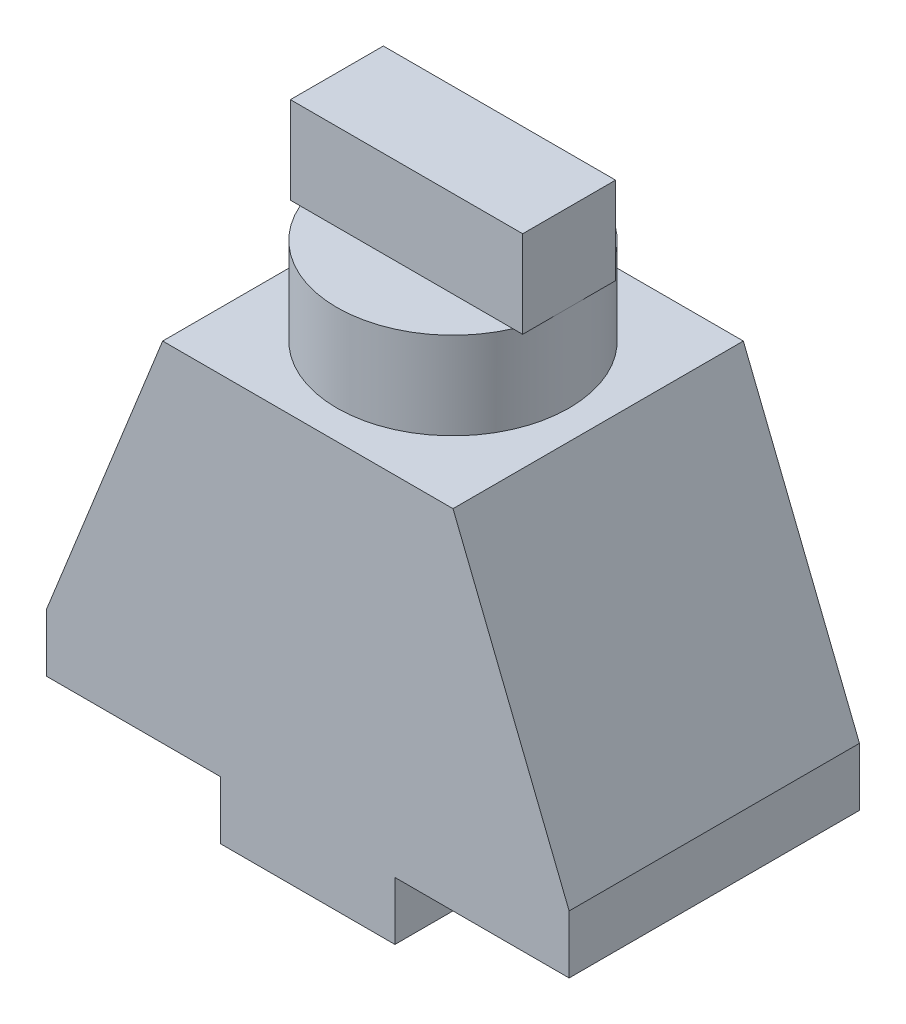
ISO-10303-21;
HEADER;
FILE_DESCRIPTION(('STEP AP214'),'2;1');
FILE_NAME('part.step','',(''),(''),'','','');
FILE_SCHEMA(('AUTOMOTIVE_DESIGN { 1 0 10303 214 1 1 1 1 }'));
ENDSEC;
DATA;
#1=APPLICATION_CONTEXT('core data for automotive mechanical design processes');
#2=APPLICATION_PROTOCOL_DEFINITION('international standard','automotive_design',2000,#1);
#3=PRODUCT_CONTEXT('',#1,'mechanical');
#4=PRODUCT('Part','Part','',(#3));
#5=PRODUCT_RELATED_PRODUCT_CATEGORY('part','',(#4));
#6=PRODUCT_DEFINITION_FORMATION('','',#4);
#7=PRODUCT_DEFINITION_CONTEXT('part definition',#1,'design');
#8=PRODUCT_DEFINITION('design','',#6,#7);
#9=PRODUCT_DEFINITION_SHAPE('','',#8);
#10=(LENGTH_UNIT() NAMED_UNIT(*) SI_UNIT(.MILLI.,.METRE.));
#11=(NAMED_UNIT(*) PLANE_ANGLE_UNIT() SI_UNIT($,.RADIAN.));
#12=(NAMED_UNIT(*) SI_UNIT($,.STERADIAN.) SOLID_ANGLE_UNIT());
#13=UNCERTAINTY_MEASURE_WITH_UNIT(LENGTH_MEASURE(1.E-05),#10,'distance_accuracy_value','');
#14=(GEOMETRIC_REPRESENTATION_CONTEXT(3) GLOBAL_UNCERTAINTY_ASSIGNED_CONTEXT((#13)) GLOBAL_UNIT_ASSIGNED_CONTEXT((#10,
#11,#12)) REPRESENTATION_CONTEXT('',''));
#15=CARTESIAN_POINT('',(0.,0.,0.));
#16=DIRECTION('',(0.,0.,1.));
#17=DIRECTION('',(1.,0.,0.));
#18=AXIS2_PLACEMENT_3D('',#15,#16,#17);
#19=CARTESIAN_POINT('',(0.,70.,25.));
#20=DIRECTION('',(0.,1.,0.));
#21=DIRECTION('',(0.,0.,1.));
#22=AXIS2_PLACEMENT_3D('',#19,#20,#21);
#23=PLANE('',#22);
#24=DIRECTION('',(1.,0.,0.));
#25=VECTOR('',#24,1.);
#26=CARTESIAN_POINT('',(-20.,70.,33.));
#27=LINE('',#26,#25);
#28=CARTESIAN_POINT('',(-18.3303027798234,70.,33.));
#29=VERTEX_POINT('',#28);
#30=CARTESIAN_POINT('',(18.3303027798234,70.,33.));
#31=VERTEX_POINT('',#30);
#32=EDGE_CURVE('E12',#29,#31,#27,.T.);
#33=ORIENTED_EDGE('',*,*,#32,.F.);
#34=CARTESIAN_POINT('',(0.,70.,25.));
#35=DIRECTION('',(0.,1.,0.));
#36=DIRECTION('',(0.,0.,1.));
#37=AXIS2_PLACEMENT_3D('',#34,#35,#36);
#38=CIRCLE('',#37,20.);
#39=EDGE_CURVE('E267',#29,#31,#38,.T.);
#40=ORIENTED_EDGE('',*,*,#39,.T.);
#41=EDGE_LOOP('',(#33,#40));
#42=FACE_BOUND('',#41,.T.);
#43=ADVANCED_FACE('F47',(#42),#23,.T.);
#44=CARTESIAN_POINT('',(45.,5.,50.));
#45=DIRECTION('',(-1.,0.,0.));
#46=DIRECTION('',(0.,0.,1.));
#47=AXIS2_PLACEMENT_3D('',#44,#45,#46);
#48=PLANE('',#47);
#49=DIRECTION('',(0.,1.,0.));
#50=VECTOR('',#49,1.);
#51=CARTESIAN_POINT('',(45.,5.,0.));
#52=LINE('',#51,#50);
#53=CARTESIAN_POINT('',(45.,-5.,0.));
#54=VERTEX_POINT('',#53);
#55=CARTESIAN_POINT('',(45.,5.00000000000001,0.));
#56=VERTEX_POINT('',#55);
#57=EDGE_CURVE('E355',#54,#56,#52,.T.);
#58=ORIENTED_EDGE('',*,*,#57,.T.);
#59=DIRECTION('',(0.,0.,1.));
#60=VECTOR('',#59,1.);
#61=CARTESIAN_POINT('',(45.,5.00000000000001,0.));
#62=LINE('',#61,#60);
#63=CARTESIAN_POINT('',(45.,5.00000000000001,50.));
#64=VERTEX_POINT('',#63);
#65=EDGE_CURVE('E273',#64,#56,#62,.F.);
#66=ORIENTED_EDGE('',*,*,#65,.F.);
#67=DIRECTION('',(0.,1.,0.));
#68=VECTOR('',#67,1.);
#69=CARTESIAN_POINT('',(45.,5.,50.));
#70=LINE('',#69,#68);
#71=CARTESIAN_POINT('',(45.,-5.,50.));
#72=VERTEX_POINT('',#71);
#73=EDGE_CURVE('E358',#72,#64,#70,.T.);
#74=ORIENTED_EDGE('',*,*,#73,.F.);
#75=DIRECTION('',(0.,0.,-1.));
#76=VECTOR('',#75,1.);
#77=CARTESIAN_POINT('',(45.,-5.,50.));
#78=LINE('',#77,#76);
#79=EDGE_CURVE('E446',#72,#54,#78,.T.);
#80=ORIENTED_EDGE('',*,*,#79,.T.);
#81=EDGE_LOOP('',(#58,#66,#74,#80));
#82=FACE_BOUND('',#81,.T.);
#83=ADVANCED_FACE('F51',(#82),#48,.F.);
#84=CARTESIAN_POINT('',(-45.,5.,50.));
#85=DIRECTION('',(1.,0.,0.));
#86=DIRECTION('',(0.,0.,-1.));
#87=AXIS2_PLACEMENT_3D('',#84,#85,#86);
#88=PLANE('',#87);
#89=DIRECTION('',(0.,-1.,0.));
#90=VECTOR('',#89,1.);
#91=CARTESIAN_POINT('',(-45.,5.,0.));
#92=LINE('',#91,#90);
#93=CARTESIAN_POINT('',(-45.,5.,0.));
#94=VERTEX_POINT('',#93);
#95=CARTESIAN_POINT('',(-45.,-5.,0.));
#96=VERTEX_POINT('',#95);
#97=EDGE_CURVE('E347',#94,#96,#92,.T.);
#98=ORIENTED_EDGE('',*,*,#97,.T.);
#99=DIRECTION('',(0.,0.,-1.));
#100=VECTOR('',#99,1.);
#101=CARTESIAN_POINT('',(-45.,-5.,50.));
#102=LINE('',#101,#100);
#103=CARTESIAN_POINT('',(-45.,-5.,50.));
#104=VERTEX_POINT('',#103);
#105=EDGE_CURVE('E333',#104,#96,#102,.T.);
#106=ORIENTED_EDGE('',*,*,#105,.F.);
#107=DIRECTION('',(0.,-1.,0.));
#108=VECTOR('',#107,1.);
#109=CARTESIAN_POINT('',(-45.,5.,50.));
#110=LINE('',#109,#108);
#111=CARTESIAN_POINT('',(-45.,4.99999999999999,50.));
#112=VERTEX_POINT('',#111);
#113=EDGE_CURVE('E353',#112,#104,#110,.T.);
#114=ORIENTED_EDGE('',*,*,#113,.F.);
#115=DIRECTION('',(0.,0.,-1.));
#116=VECTOR('',#115,1.);
#117=CARTESIAN_POINT('',(-45.,5.,50.));
#118=LINE('',#117,#116);
#119=EDGE_CURVE('E52',#112,#94,#118,.T.);
#120=ORIENTED_EDGE('',*,*,#119,.T.);
#121=EDGE_LOOP('',(#98,#106,#114,#120));
#122=FACE_BOUND('',#121,.T.);
#123=ADVANCED_FACE('F492',(#122),#88,.F.);
#124=CARTESIAN_POINT('',(-45.,-5.,50.));
#125=DIRECTION('',(0.,1.,0.));
#126=DIRECTION('',(0.,0.,1.));
#127=AXIS2_PLACEMENT_3D('',#124,#125,#126);
#128=PLANE('',#127);
#129=DIRECTION('',(1.,0.,0.));
#130=VECTOR('',#129,1.);
#131=CARTESIAN_POINT('',(-45.,-5.,0.));
#132=LINE('',#131,#130);
#133=CARTESIAN_POINT('',(-15.,-5.,0.));
#134=VERTEX_POINT('',#133);
#135=EDGE_CURVE('E352',#96,#134,#132,.T.);
#136=ORIENTED_EDGE('',*,*,#135,.T.);
#137=DIRECTION('',(0.,0.,-1.));
#138=VECTOR('',#137,1.);
#139=CARTESIAN_POINT('',(-15.,-5.,50.));
#140=LINE('',#139,#138);
#141=CARTESIAN_POINT('',(-15.,-5.,50.));
#142=VERTEX_POINT('',#141);
#143=EDGE_CURVE('E336',#142,#134,#140,.T.);
#144=ORIENTED_EDGE('',*,*,#143,.F.);
#145=DIRECTION('',(1.,0.,0.));
#146=VECTOR('',#145,1.);
#147=CARTESIAN_POINT('',(-45.,-5.,50.));
#148=LINE('',#147,#146);
#149=EDGE_CURVE('E351',#104,#142,#148,.T.);
#150=ORIENTED_EDGE('',*,*,#149,.F.);
#151=ORIENTED_EDGE('',*,*,#105,.T.);
#152=EDGE_LOOP('',(#136,#144,#150,#151));
#153=FACE_BOUND('',#152,.T.);
#154=ADVANCED_FACE('F481',(#153),#128,.F.);
#155=CARTESIAN_POINT('',(-15.,-5.,50.));
#156=DIRECTION('',(1.,0.,0.));
#157=DIRECTION('',(0.,0.,-1.));
#158=AXIS2_PLACEMENT_3D('',#155,#156,#157);
#159=PLANE('',#158);
#160=DIRECTION('',(0.,-1.,0.));
#161=VECTOR('',#160,1.);
#162=CARTESIAN_POINT('',(-15.,-5.,0.));
#163=LINE('',#162,#161);
#164=CARTESIAN_POINT('',(-15.,-15.,0.));
#165=VERTEX_POINT('',#164);
#166=EDGE_CURVE('E476',#134,#165,#163,.T.);
#167=ORIENTED_EDGE('',*,*,#166,.T.);
#168=DIRECTION('',(0.,0.,-1.));
#169=VECTOR('',#168,1.);
#170=CARTESIAN_POINT('',(-15.,-15.,50.));
#171=LINE('',#170,#169);
#172=CARTESIAN_POINT('',(-15.,-15.,50.));
#173=VERTEX_POINT('',#172);
#174=EDGE_CURVE('E343',#173,#165,#171,.T.);
#175=ORIENTED_EDGE('',*,*,#174,.F.);
#176=DIRECTION('',(0.,-1.,0.));
#177=VECTOR('',#176,1.);
#178=CARTESIAN_POINT('',(-15.,-5.,50.));
#179=LINE('',#178,#177);
#180=EDGE_CURVE('E483',#142,#173,#179,.T.);
#181=ORIENTED_EDGE('',*,*,#180,.F.);
#182=ORIENTED_EDGE('',*,*,#143,.T.);
#183=EDGE_LOOP('',(#167,#175,#181,#182));
#184=FACE_BOUND('',#183,.T.);
#185=ADVANCED_FACE('F488',(#184),#159,.F.);
#186=CARTESIAN_POINT('',(-15.,-15.,50.));
#187=DIRECTION('',(0.,1.,0.));
#188=DIRECTION('',(0.,0.,1.));
#189=AXIS2_PLACEMENT_3D('',#186,#187,#188);
#190=PLANE('',#189);
#191=DIRECTION('',(1.,0.,0.));
#192=VECTOR('',#191,1.);
#193=CARTESIAN_POINT('',(-15.,-15.,0.));
#194=LINE('',#193,#192);
#195=CARTESIAN_POINT('',(15.,-15.,0.));
#196=VERTEX_POINT('',#195);
#197=EDGE_CURVE('E460',#165,#196,#194,.T.);
#198=ORIENTED_EDGE('',*,*,#197,.T.);
#199=DIRECTION('',(0.,0.,-1.));
#200=VECTOR('',#199,1.);
#201=CARTESIAN_POINT('',(15.,-15.,50.));
#202=LINE('',#201,#200);
#203=CARTESIAN_POINT('',(15.,-15.,50.));
#204=VERTEX_POINT('',#203);
#205=EDGE_CURVE('E464',#204,#196,#202,.T.);
#206=ORIENTED_EDGE('',*,*,#205,.F.);
#207=DIRECTION('',(1.,0.,0.));
#208=VECTOR('',#207,1.);
#209=CARTESIAN_POINT('',(-15.,-15.,50.));
#210=LINE('',#209,#208);
#211=EDGE_CURVE('E475',#173,#204,#210,.T.);
#212=ORIENTED_EDGE('',*,*,#211,.F.);
#213=ORIENTED_EDGE('',*,*,#174,.T.);
#214=EDGE_LOOP('',(#198,#206,#212,#213));
#215=FACE_BOUND('',#214,.T.);
#216=ADVANCED_FACE('F468',(#215),#190,.F.);
#217=CARTESIAN_POINT('',(15.,-5.,50.));
#218=DIRECTION('',(-1.,0.,0.));
#219=DIRECTION('',(0.,0.,1.));
#220=AXIS2_PLACEMENT_3D('',#217,#218,#219);
#221=PLANE('',#220);
#222=DIRECTION('',(0.,1.,0.));
#223=VECTOR('',#222,1.);
#224=CARTESIAN_POINT('',(15.,-5.,0.));
#225=LINE('',#224,#223);
#226=CARTESIAN_POINT('',(15.,-5.,0.));
#227=VERTEX_POINT('',#226);
#228=EDGE_CURVE('E454',#196,#227,#225,.T.);
#229=ORIENTED_EDGE('',*,*,#228,.T.);
#230=DIRECTION('',(0.,0.,-1.));
#231=VECTOR('',#230,1.);
#232=CARTESIAN_POINT('',(15.,-5.,50.));
#233=LINE('',#232,#231);
#234=CARTESIAN_POINT('',(15.,-5.,50.));
#235=VERTEX_POINT('',#234);
#236=EDGE_CURVE('E465',#235,#227,#233,.T.);
#237=ORIENTED_EDGE('',*,*,#236,.F.);
#238=DIRECTION('',(0.,1.,0.));
#239=VECTOR('',#238,1.);
#240=CARTESIAN_POINT('',(15.,-5.,50.));
#241=LINE('',#240,#239);
#242=EDGE_CURVE('E482',#204,#235,#241,.T.);
#243=ORIENTED_EDGE('',*,*,#242,.F.);
#244=ORIENTED_EDGE('',*,*,#205,.T.);
#245=EDGE_LOOP('',(#229,#237,#243,#244));
#246=FACE_BOUND('',#245,.T.);
#247=ADVANCED_FACE('F491',(#246),#221,.F.);
#248=CARTESIAN_POINT('',(15.,-5.,50.));
#249=DIRECTION('',(0.,1.,0.));
#250=DIRECTION('',(0.,0.,1.));
#251=AXIS2_PLACEMENT_3D('',#248,#249,#250);
#252=PLANE('',#251);
#253=DIRECTION('',(1.,0.,0.));
#254=VECTOR('',#253,1.);
#255=CARTESIAN_POINT('',(15.,-5.,0.));
#256=LINE('',#255,#254);
#257=EDGE_CURVE('E360',#227,#54,#256,.T.);
#258=ORIENTED_EDGE('',*,*,#257,.T.);
#259=ORIENTED_EDGE('',*,*,#79,.F.);
#260=DIRECTION('',(1.,0.,0.));
#261=VECTOR('',#260,1.);
#262=CARTESIAN_POINT('',(15.,-5.,50.));
#263=LINE('',#262,#261);
#264=EDGE_CURVE('E444',#235,#72,#263,.T.);
#265=ORIENTED_EDGE('',*,*,#264,.F.);
#266=ORIENTED_EDGE('',*,*,#236,.T.);
#267=EDGE_LOOP('',(#258,#259,#265,#266));
#268=FACE_BOUND('',#267,.T.);
#269=ADVANCED_FACE('F317',(#268),#252,.F.);
#270=CARTESIAN_POINT('',(0.,0.,50.));
#271=DIRECTION('',(0.,0.,1.));
#272=DIRECTION('',(1.,0.,0.));
#273=AXIS2_PLACEMENT_3D('',#270,#271,#272);
#274=PLANE('',#273);
#275=ORIENTED_EDGE('',*,*,#73,.T.);
#276=DIRECTION('',(0.371390676354104,-0.928476690885259,0.));
#277=VECTOR('',#276,1.);
#278=CARTESIAN_POINT('',(25.,55.,50.));
#279=LINE('',#278,#277);
#280=CARTESIAN_POINT('',(25.,55.,50.));
#281=VERTEX_POINT('',#280);
#282=EDGE_CURVE('E282',#281,#64,#279,.T.);
#283=ORIENTED_EDGE('',*,*,#282,.F.);
#284=DIRECTION('',(1.,0.,0.));
#285=VECTOR('',#284,1.);
#286=CARTESIAN_POINT('',(-25.,55.,50.));
#287=LINE('',#286,#285);
#288=CARTESIAN_POINT('',(-25.,55.,50.));
#289=VERTEX_POINT('',#288);
#290=EDGE_CURVE('E382',#289,#281,#287,.T.);
#291=ORIENTED_EDGE('',*,*,#290,.F.);
#292=DIRECTION('',(-0.371390676354104,-0.928476690885259,0.));
#293=VECTOR('',#292,1.);
#294=CARTESIAN_POINT('',(-25.,55.,50.));
#295=LINE('',#294,#293);
#296=EDGE_CURVE('E365',#289,#112,#295,.T.);
#297=ORIENTED_EDGE('',*,*,#296,.T.);
#298=ORIENTED_EDGE('',*,*,#113,.T.);
#299=ORIENTED_EDGE('',*,*,#149,.T.);
#300=ORIENTED_EDGE('',*,*,#180,.T.);
#301=ORIENTED_EDGE('',*,*,#211,.T.);
#302=ORIENTED_EDGE('',*,*,#242,.T.);
#303=ORIENTED_EDGE('',*,*,#264,.T.);
#304=EDGE_LOOP('',(#275,#283,#291,#297,#298,#299,#300,#301,#302,#303));
#305=FACE_BOUND('',#304,.T.);
#306=ADVANCED_FACE('F311',(#305),#274,.T.);
#307=CARTESIAN_POINT('',(0.,0.,0.));
#308=DIRECTION('',(0.,0.,1.));
#309=DIRECTION('',(1.,0.,0.));
#310=AXIS2_PLACEMENT_3D('',#307,#308,#309);
#311=PLANE('',#310);
#312=ORIENTED_EDGE('',*,*,#57,.F.);
#313=ORIENTED_EDGE('',*,*,#257,.F.);
#314=ORIENTED_EDGE('',*,*,#228,.F.);
#315=ORIENTED_EDGE('',*,*,#197,.F.);
#316=ORIENTED_EDGE('',*,*,#166,.F.);
#317=ORIENTED_EDGE('',*,*,#135,.F.);
#318=ORIENTED_EDGE('',*,*,#97,.F.);
#319=DIRECTION('',(-0.371390676354103,-0.92847669088526,0.));
#320=VECTOR('',#319,1.);
#321=CARTESIAN_POINT('',(-25.,55.,0.));
#322=LINE('',#321,#320);
#323=CARTESIAN_POINT('',(-25.,55.,0.));
#324=VERTEX_POINT('',#323);
#325=EDGE_CURVE('E276',#324,#94,#322,.T.);
#326=ORIENTED_EDGE('',*,*,#325,.F.);
#327=DIRECTION('',(-1.,0.,0.));
#328=VECTOR('',#327,1.);
#329=CARTESIAN_POINT('',(-25.,55.,0.));
#330=LINE('',#329,#328);
#331=CARTESIAN_POINT('',(25.,55.,0.));
#332=VERTEX_POINT('',#331);
#333=EDGE_CURVE('E278',#332,#324,#330,.T.);
#334=ORIENTED_EDGE('',*,*,#333,.F.);
#335=DIRECTION('',(0.371390676354104,-0.928476690885259,0.));
#336=VECTOR('',#335,1.);
#337=CARTESIAN_POINT('',(25.,55.,0.));
#338=LINE('',#337,#336);
#339=EDGE_CURVE('E277',#332,#56,#338,.T.);
#340=ORIENTED_EDGE('',*,*,#339,.T.);
#341=EDGE_LOOP('',(#312,#313,#314,#315,#316,#317,#318,#326,#334,#340));
#342=FACE_BOUND('',#341,.T.);
#343=ADVANCED_FACE('F314',(#342),#311,.F.);
#344=CARTESIAN_POINT('',(0.,55.,0.));
#345=DIRECTION('',(0.,1.,0.));
#346=DIRECTION('',(0.,0.,1.));
#347=AXIS2_PLACEMENT_3D('',#344,#345,#346);
#348=PLANE('',#347);
#349=CARTESIAN_POINT('',(0.,55.,25.));
#350=DIRECTION('',(0.,1.,0.));
#351=DIRECTION('',(0.,0.,1.));
#352=AXIS2_PLACEMENT_3D('',#349,#350,#351);
#353=CIRCLE('',#352,20.);
#354=CARTESIAN_POINT('',(0.,55.,45.));
#355=VERTEX_POINT('',#354);
#356=EDGE_CURVE('E275',#355,#355,#353,.T.);
#357=ORIENTED_EDGE('',*,*,#356,.F.);
#358=EDGE_LOOP('',(#357));
#359=FACE_BOUND('',#358,.T.);
#360=DIRECTION('',(0.,0.,-1.));
#361=VECTOR('',#360,1.);
#362=CARTESIAN_POINT('',(25.,55.,0.));
#363=LINE('',#362,#361);
#364=EDGE_CURVE('E266',#281,#332,#363,.T.);
#365=ORIENTED_EDGE('',*,*,#364,.T.);
#366=ORIENTED_EDGE('',*,*,#333,.T.);
#367=DIRECTION('',(0.,0.,1.));
#368=VECTOR('',#367,1.);
#369=CARTESIAN_POINT('',(-25.,55.,0.));
#370=LINE('',#369,#368);
#371=EDGE_CURVE('E380',#324,#289,#370,.T.);
#372=ORIENTED_EDGE('',*,*,#371,.T.);
#373=ORIENTED_EDGE('',*,*,#290,.T.);
#374=EDGE_LOOP('',(#365,#366,#372,#373));
#375=FACE_BOUND('',#374,.T.);
#376=ADVANCED_FACE('F379',(#359,#375),#348,.T.);
#377=CARTESIAN_POINT('',(-40.5172413793104,16.2068965517241,0.));
#378=DIRECTION('',(0.92847669088526,-0.371390676354103,0.));
#379=DIRECTION('',(0.371390676354103,0.92847669088526,0.));
#380=AXIS2_PLACEMENT_3D('',#377,#378,#379);
#381=PLANE('',#380);
#382=DIRECTION('',(0.,0.,-1.));
#383=VECTOR('',#382,1.);
#384=CARTESIAN_POINT('',(-29.0852974398952,44.7867564002622,10.));
#385=LINE('',#384,#383);
#386=CARTESIAN_POINT('',(-29.0852974398952,44.7867564002622,40.));
#387=VERTEX_POINT('',#386);
#388=CARTESIAN_POINT('',(-29.0852974398952,44.7867564002622,10.));
#389=VERTEX_POINT('',#388);
#390=EDGE_CURVE('E223',#387,#389,#385,.T.);
#391=ORIENTED_EDGE('',*,*,#390,.F.);
#392=DIRECTION('',(0.371390676354104,0.92847669088526,0.));
#393=VECTOR('',#392,1.);
#394=CARTESIAN_POINT('',(-29.0852974398952,44.7867564002622,40.));
#395=LINE('',#394,#393);
#396=CARTESIAN_POINT('',(-39.8556270541642,17.8609323645896,40.));
#397=VERTEX_POINT('',#396);
#398=EDGE_CURVE('E68',#397,#387,#395,.T.);
#399=ORIENTED_EDGE('',*,*,#398,.F.);
#400=DIRECTION('',(0.,0.,1.));
#401=VECTOR('',#400,1.);
#402=CARTESIAN_POINT('',(-39.8556270541642,17.8609323645896,10.));
#403=LINE('',#402,#401);
#404=CARTESIAN_POINT('',(-39.8556270541642,17.8609323645896,10.));
#405=VERTEX_POINT('',#404);
#406=EDGE_CURVE('E211',#405,#397,#403,.T.);
#407=ORIENTED_EDGE('',*,*,#406,.F.);
#408=DIRECTION('',(-0.371390676354104,-0.92847669088526,0.));
#409=VECTOR('',#408,1.);
#410=CARTESIAN_POINT('',(-29.0852974398952,44.7867564002622,10.));
#411=LINE('',#410,#409);
#412=EDGE_CURVE('E220',#389,#405,#411,.T.);
#413=ORIENTED_EDGE('',*,*,#412,.F.);
#414=EDGE_LOOP('',(#391,#399,#407,#413));
#415=FACE_BOUND('',#414,.T.);
#416=ORIENTED_EDGE('',*,*,#325,.T.);
#417=ORIENTED_EDGE('',*,*,#119,.F.);
#418=ORIENTED_EDGE('',*,*,#296,.F.);
#419=ORIENTED_EDGE('',*,*,#371,.F.);
#420=EDGE_LOOP('',(#416,#417,#418,#419));
#421=FACE_BOUND('',#420,.T.);
#422=ADVANCED_FACE('F308',(#415,#421),#381,.F.);
#423=CARTESIAN_POINT('',(40.5172413793104,16.2068965517241,0.));
#424=DIRECTION('',(0.92847669088526,0.371390676354104,0.));
#425=DIRECTION('',(-0.371390676354104,0.928476690885259,0.));
#426=AXIS2_PLACEMENT_3D('',#423,#424,#425);
#427=PLANE('',#426);
#428=ORIENTED_EDGE('',*,*,#282,.T.);
#429=ORIENTED_EDGE('',*,*,#65,.T.);
#430=ORIENTED_EDGE('',*,*,#339,.F.);
#431=ORIENTED_EDGE('',*,*,#364,.F.);
#432=EDGE_LOOP('',(#428,#429,#430,#431));
#433=FACE_BOUND('',#432,.T.);
#434=ADVANCED_FACE('F300',(#433),#427,.T.);
#435=CARTESIAN_POINT('',(0.,70.,25.));
#436=DIRECTION('',(0.,-1.,0.));
#437=DIRECTION('',(0.,0.,-1.));
#438=AXIS2_PLACEMENT_3D('',#435,#436,#437);
#439=CYLINDRICAL_SURFACE('',#438,20.);
#440=CARTESIAN_POINT('',(20.,70.,25.));
#441=VERTEX_POINT('',#440);
#442=EDGE_CURVE('E270',#31,#441,#38,.T.);
#443=ORIENTED_EDGE('',*,*,#442,.F.);
#444=ORIENTED_EDGE('',*,*,#39,.F.);
#445=CARTESIAN_POINT('',(-20.,70.,25.));
#446=VERTEX_POINT('',#445);
#447=EDGE_CURVE('E536',#446,#29,#38,.T.);
#448=ORIENTED_EDGE('',*,*,#447,.F.);
#449=CARTESIAN_POINT('',(-18.3303027798234,70.,17.));
#450=VERTEX_POINT('',#449);
#451=EDGE_CURVE('E522',#450,#446,#38,.T.);
#452=ORIENTED_EDGE('',*,*,#451,.F.);
#453=CARTESIAN_POINT('',(18.3303027798234,70.,17.));
#454=VERTEX_POINT('',#453);
#455=EDGE_CURVE('E520',#454,#450,#38,.T.);
#456=ORIENTED_EDGE('',*,*,#455,.F.);
#457=EDGE_CURVE('E272',#441,#454,#38,.T.);
#458=ORIENTED_EDGE('',*,*,#457,.F.);
#459=EDGE_LOOP('',(#443,#444,#448,#452,#456,#458));
#460=FACE_BOUND('',#459,.T.);
#461=ORIENTED_EDGE('',*,*,#356,.T.);
#462=EDGE_LOOP('',(#461));
#463=FACE_BOUND('',#462,.T.);
#464=ADVANCED_FACE('F310',(#460,#463),#439,.T.);
#465=DIRECTION('',(-1.,0.,0.));
#466=VECTOR('',#465,1.);
#467=CARTESIAN_POINT('',(-20.,70.,17.));
#468=LINE('',#467,#466);
#469=EDGE_CURVE('E59',#454,#450,#468,.T.);
#470=ORIENTED_EDGE('',*,*,#469,.F.);
#471=ORIENTED_EDGE('',*,*,#455,.T.);
#472=EDGE_LOOP('',(#470,#471));
#473=FACE_BOUND('',#472,.T.);
#474=ADVANCED_FACE('F498',(#473),#23,.T.);
#475=CARTESIAN_POINT('',(0.,70.,0.));
#476=DIRECTION('',(0.,1.,0.));
#477=DIRECTION('',(0.,0.,1.));
#478=AXIS2_PLACEMENT_3D('',#475,#476,#477);
#479=PLANE('',#478);
#480=CARTESIAN_POINT('',(20.,70.,33.));
#481=VERTEX_POINT('',#480);
#482=EDGE_CURVE('E62',#31,#481,#27,.T.);
#483=ORIENTED_EDGE('',*,*,#482,.F.);
#484=ORIENTED_EDGE('',*,*,#442,.T.);
#485=DIRECTION('',(0.,0.,-1.));
#486=VECTOR('',#485,1.);
#487=CARTESIAN_POINT('',(20.,70.,17.));
#488=LINE('',#487,#486);
#489=EDGE_CURVE('E243',#481,#441,#488,.T.);
#490=ORIENTED_EDGE('',*,*,#489,.F.);
#491=EDGE_LOOP('',(#483,#484,#490));
#492=FACE_BOUND('',#491,.T.);
#493=ADVANCED_FACE('F504',(#492),#479,.F.);
#494=CARTESIAN_POINT('',(20.,70.,17.));
#495=VERTEX_POINT('',#494);
#496=EDGE_CURVE('E230',#441,#495,#488,.T.);
#497=ORIENTED_EDGE('',*,*,#496,.F.);
#498=ORIENTED_EDGE('',*,*,#457,.T.);
#499=EDGE_CURVE('E250',#495,#454,#468,.T.);
#500=ORIENTED_EDGE('',*,*,#499,.F.);
#501=EDGE_LOOP('',(#497,#498,#500));
#502=FACE_BOUND('',#501,.T.);
#503=ADVANCED_FACE('F509',(#502),#479,.F.);
#504=CARTESIAN_POINT('',(-20.,70.,17.));
#505=VERTEX_POINT('',#504);
#506=EDGE_CURVE('E246',#450,#505,#468,.T.);
#507=ORIENTED_EDGE('',*,*,#506,.F.);
#508=ORIENTED_EDGE('',*,*,#451,.T.);
#509=DIRECTION('',(0.,0.,1.));
#510=VECTOR('',#509,1.);
#511=CARTESIAN_POINT('',(-20.,70.,17.));
#512=LINE('',#511,#510);
#513=EDGE_CURVE('E252',#505,#446,#512,.T.);
#514=ORIENTED_EDGE('',*,*,#513,.F.);
#515=EDGE_LOOP('',(#507,#508,#514));
#516=FACE_BOUND('',#515,.T.);
#517=ADVANCED_FACE('F552',(#516),#479,.F.);
#518=CARTESIAN_POINT('',(-20.,70.,33.));
#519=VERTEX_POINT('',#518);
#520=EDGE_CURVE('E249',#446,#519,#512,.T.);
#521=ORIENTED_EDGE('',*,*,#520,.F.);
#522=ORIENTED_EDGE('',*,*,#447,.T.);
#523=EDGE_CURVE('E58',#519,#29,#27,.T.);
#524=ORIENTED_EDGE('',*,*,#523,.F.);
#525=EDGE_LOOP('',(#521,#522,#524));
#526=FACE_BOUND('',#525,.T.);
#527=ADVANCED_FACE('F514',(#526),#479,.F.);
#528=CARTESIAN_POINT('',(20.,85.,17.));
#529=DIRECTION('',(-1.,0.,0.));
#530=DIRECTION('',(0.,0.,1.));
#531=AXIS2_PLACEMENT_3D('',#528,#529,#530);
#532=PLANE('',#531);
#533=ORIENTED_EDGE('',*,*,#489,.T.);
#534=ORIENTED_EDGE('',*,*,#496,.T.);
#535=DIRECTION('',(0.,-1.,0.));
#536=VECTOR('',#535,1.);
#537=CARTESIAN_POINT('',(20.,85.,17.));
#538=LINE('',#537,#536);
#539=CARTESIAN_POINT('',(20.,85.,17.));
#540=VERTEX_POINT('',#539);
#541=EDGE_CURVE('E263',#540,#495,#538,.T.);
#542=ORIENTED_EDGE('',*,*,#541,.F.);
#543=DIRECTION('',(0.,0.,-1.));
#544=VECTOR('',#543,1.);
#545=CARTESIAN_POINT('',(20.,85.,17.));
#546=LINE('',#545,#544);
#547=CARTESIAN_POINT('',(20.,85.,33.));
#548=VERTEX_POINT('',#547);
#549=EDGE_CURVE('E231',#548,#540,#546,.T.);
#550=ORIENTED_EDGE('',*,*,#549,.F.);
#551=DIRECTION('',(0.,-1.,0.));
#552=VECTOR('',#551,1.);
#553=CARTESIAN_POINT('',(20.,85.,33.));
#554=LINE('',#553,#552);
#555=EDGE_CURVE('E245',#548,#481,#554,.T.);
#556=ORIENTED_EDGE('',*,*,#555,.T.);
#557=EDGE_LOOP('',(#533,#534,#542,#550,#556));
#558=FACE_BOUND('',#557,.T.);
#559=ADVANCED_FACE('F534',(#558),#532,.F.);
#560=CARTESIAN_POINT('',(-20.,85.,17.));
#561=DIRECTION('',(0.,0.,1.));
#562=DIRECTION('',(1.,0.,0.));
#563=AXIS2_PLACEMENT_3D('',#560,#561,#562);
#564=PLANE('',#563);
#565=ORIENTED_EDGE('',*,*,#499,.T.);
#566=ORIENTED_EDGE('',*,*,#469,.T.);
#567=ORIENTED_EDGE('',*,*,#506,.T.);
#568=DIRECTION('',(0.,-1.,0.));
#569=VECTOR('',#568,1.);
#570=CARTESIAN_POINT('',(-20.,85.,17.));
#571=LINE('',#570,#569);
#572=CARTESIAN_POINT('',(-20.,85.,17.));
#573=VERTEX_POINT('',#572);
#574=EDGE_CURVE('E258',#573,#505,#571,.T.);
#575=ORIENTED_EDGE('',*,*,#574,.F.);
#576=DIRECTION('',(-1.,0.,0.));
#577=VECTOR('',#576,1.);
#578=CARTESIAN_POINT('',(-20.,85.,17.));
#579=LINE('',#578,#577);
#580=EDGE_CURVE('E236',#540,#573,#579,.T.);
#581=ORIENTED_EDGE('',*,*,#580,.F.);
#582=ORIENTED_EDGE('',*,*,#541,.T.);
#583=EDGE_LOOP('',(#565,#566,#567,#575,#581,#582));
#584=FACE_BOUND('',#583,.T.);
#585=ADVANCED_FACE('F529',(#584),#564,.F.);
#586=CARTESIAN_POINT('',(-20.,85.,17.));
#587=DIRECTION('',(1.,0.,0.));
#588=DIRECTION('',(0.,0.,-1.));
#589=AXIS2_PLACEMENT_3D('',#586,#587,#588);
#590=PLANE('',#589);
#591=ORIENTED_EDGE('',*,*,#513,.T.);
#592=ORIENTED_EDGE('',*,*,#520,.T.);
#593=DIRECTION('',(0.,-1.,0.));
#594=VECTOR('',#593,1.);
#595=CARTESIAN_POINT('',(-20.,85.,33.));
#596=LINE('',#595,#594);
#597=CARTESIAN_POINT('',(-20.,85.,33.));
#598=VERTEX_POINT('',#597);
#599=EDGE_CURVE('E260',#598,#519,#596,.T.);
#600=ORIENTED_EDGE('',*,*,#599,.F.);
#601=DIRECTION('',(0.,0.,1.));
#602=VECTOR('',#601,1.);
#603=CARTESIAN_POINT('',(-20.,85.,17.));
#604=LINE('',#603,#602);
#605=EDGE_CURVE('E238',#573,#598,#604,.T.);
#606=ORIENTED_EDGE('',*,*,#605,.F.);
#607=ORIENTED_EDGE('',*,*,#574,.T.);
#608=EDGE_LOOP('',(#591,#592,#600,#606,#607));
#609=FACE_BOUND('',#608,.T.);
#610=ADVANCED_FACE('F549',(#609),#590,.F.);
#611=CARTESIAN_POINT('',(-20.,85.,33.));
#612=DIRECTION('',(0.,0.,-1.));
#613=DIRECTION('',(-1.,0.,0.));
#614=AXIS2_PLACEMENT_3D('',#611,#612,#613);
#615=PLANE('',#614);
#616=ORIENTED_EDGE('',*,*,#523,.T.);
#617=ORIENTED_EDGE('',*,*,#32,.T.);
#618=ORIENTED_EDGE('',*,*,#482,.T.);
#619=ORIENTED_EDGE('',*,*,#555,.F.);
#620=DIRECTION('',(1.,0.,0.));
#621=VECTOR('',#620,1.);
#622=CARTESIAN_POINT('',(-20.,85.,33.));
#623=LINE('',#622,#621);
#624=EDGE_CURVE('E239',#598,#548,#623,.T.);
#625=ORIENTED_EDGE('',*,*,#624,.F.);
#626=ORIENTED_EDGE('',*,*,#599,.T.);
#627=EDGE_LOOP('',(#616,#617,#618,#619,#625,#626));
#628=FACE_BOUND('',#627,.T.);
#629=ADVANCED_FACE('F542',(#628),#615,.F.);
#630=CARTESIAN_POINT('',(0.,85.,0.));
#631=DIRECTION('',(0.,1.,0.));
#632=DIRECTION('',(0.,0.,1.));
#633=AXIS2_PLACEMENT_3D('',#630,#631,#632);
#634=PLANE('',#633);
#635=ORIENTED_EDGE('',*,*,#549,.T.);
#636=ORIENTED_EDGE('',*,*,#580,.T.);
#637=ORIENTED_EDGE('',*,*,#605,.T.);
#638=ORIENTED_EDGE('',*,*,#624,.T.);
#639=EDGE_LOOP('',(#635,#636,#637,#638));
#640=FACE_BOUND('',#639,.T.);
#641=ADVANCED_FACE('F557',(#640),#634,.T.);
#642=CARTESIAN_POINT('',(-15.1581470766163,39.2158962549506,40.));
#643=DIRECTION('',(0.,0.,1.));
#644=DIRECTION('',(0.,-1.,0.));
#645=AXIS2_PLACEMENT_3D('',#642,#643,#644);
#646=PLANE('',#645);
#647=ORIENTED_EDGE('',*,*,#398,.T.);
#648=DIRECTION('',(-0.928476690885259,0.371390676354104,0.));
#649=VECTOR('',#648,1.);
#650=CARTESIAN_POINT('',(-15.1581470766163,39.2158962549506,40.));
#651=LINE('',#650,#649);
#652=CARTESIAN_POINT('',(-15.1581470766163,39.2158962549506,40.));
#653=VERTEX_POINT('',#652);
#654=EDGE_CURVE('E195',#653,#387,#651,.T.);
#655=ORIENTED_EDGE('',*,*,#654,.F.);
#656=DIRECTION('',(0.371390676354104,0.92847669088526,0.));
#657=VECTOR('',#656,1.);
#658=CARTESIAN_POINT('',(-15.1581470766163,39.2158962549506,40.));
#659=LINE('',#658,#657);
#660=CARTESIAN_POINT('',(-25.9284766908853,12.2900722192781,40.));
#661=VERTEX_POINT('',#660);
#662=EDGE_CURVE('E196',#661,#653,#659,.T.);
#663=ORIENTED_EDGE('',*,*,#662,.F.);
#664=DIRECTION('',(-0.928476690885259,0.371390676354104,0.));
#665=VECTOR('',#664,1.);
#666=CARTESIAN_POINT('',(-25.9284766908853,12.2900722192781,40.));
#667=LINE('',#666,#665);
#668=EDGE_CURVE('E227',#661,#397,#667,.T.);
#669=ORIENTED_EDGE('',*,*,#668,.T.);
#670=EDGE_LOOP('',(#647,#655,#663,#669));
#671=FACE_BOUND('',#670,.T.);
#672=ADVANCED_FACE('F191',(#671),#646,.F.);
#673=CARTESIAN_POINT('',(-25.9284766908853,12.2900722192781,10.));
#674=DIRECTION('',(-0.371390676354103,-0.928476690885259,0.));
#675=DIRECTION('',(0.92847669088526,-0.371390676354104,0.));
#676=AXIS2_PLACEMENT_3D('',#673,#674,#675);
#677=PLANE('',#676);
#678=ORIENTED_EDGE('',*,*,#406,.T.);
#679=ORIENTED_EDGE('',*,*,#668,.F.);
#680=DIRECTION('',(0.,0.,1.));
#681=VECTOR('',#680,1.);
#682=CARTESIAN_POINT('',(-25.9284766908853,12.2900722192781,10.));
#683=LINE('',#682,#681);
#684=CARTESIAN_POINT('',(-25.9284766908853,12.2900722192781,10.));
#685=VERTEX_POINT('',#684);
#686=EDGE_CURVE('E205',#685,#661,#683,.T.);
#687=ORIENTED_EDGE('',*,*,#686,.F.);
#688=DIRECTION('',(-0.928476690885259,0.371390676354104,0.));
#689=VECTOR('',#688,1.);
#690=CARTESIAN_POINT('',(-25.9284766908853,12.2900722192781,10.));
#691=LINE('',#690,#689);
#692=EDGE_CURVE('E229',#685,#405,#691,.T.);
#693=ORIENTED_EDGE('',*,*,#692,.T.);
#694=EDGE_LOOP('',(#678,#679,#687,#693));
#695=FACE_BOUND('',#694,.T.);
#696=ADVANCED_FACE('F609',(#695),#677,.F.);
#697=CARTESIAN_POINT('',(-15.1581470766163,39.2158962549506,10.));
#698=DIRECTION('',(0.,0.,-1.));
#699=DIRECTION('',(0.,1.,0.));
#700=AXIS2_PLACEMENT_3D('',#697,#698,#699);
#701=PLANE('',#700);
#702=ORIENTED_EDGE('',*,*,#412,.T.);
#703=ORIENTED_EDGE('',*,*,#692,.F.);
#704=DIRECTION('',(-0.371390676354104,-0.92847669088526,0.));
#705=VECTOR('',#704,1.);
#706=CARTESIAN_POINT('',(-15.1581470766163,39.2158962549506,10.));
#707=LINE('',#706,#705);
#708=CARTESIAN_POINT('',(-15.1581470766163,39.2158962549506,10.));
#709=VERTEX_POINT('',#708);
#710=EDGE_CURVE('E208',#709,#685,#707,.T.);
#711=ORIENTED_EDGE('',*,*,#710,.F.);
#712=DIRECTION('',(-0.928476690885259,0.371390676354104,0.));
#713=VECTOR('',#712,1.);
#714=CARTESIAN_POINT('',(-15.1581470766163,39.2158962549506,10.));
#715=LINE('',#714,#713);
#716=EDGE_CURVE('E202',#709,#389,#715,.T.);
#717=ORIENTED_EDGE('',*,*,#716,.T.);
#718=EDGE_LOOP('',(#702,#703,#711,#717));
#719=FACE_BOUND('',#718,.T.);
#720=ADVANCED_FACE('F617',(#719),#701,.F.);
#721=CARTESIAN_POINT('',(-15.1581470766163,39.2158962549506,10.));
#722=DIRECTION('',(0.371390676354104,0.928476690885259,0.));
#723=DIRECTION('',(-0.928476690885259,0.371390676354104,0.));
#724=AXIS2_PLACEMENT_3D('',#721,#722,#723);
#725=PLANE('',#724);
#726=ORIENTED_EDGE('',*,*,#390,.T.);
#727=ORIENTED_EDGE('',*,*,#716,.F.);
#728=DIRECTION('',(0.,0.,-1.));
#729=VECTOR('',#728,1.);
#730=CARTESIAN_POINT('',(-15.1581470766163,39.2158962549506,10.));
#731=LINE('',#730,#729);
#732=EDGE_CURVE('E201',#653,#709,#731,.T.);
#733=ORIENTED_EDGE('',*,*,#732,.F.);
#734=ORIENTED_EDGE('',*,*,#654,.T.);
#735=EDGE_LOOP('',(#726,#727,#733,#734));
#736=FACE_BOUND('',#735,.T.);
#737=ADVANCED_FACE('F207',(#736),#725,.F.);
#738=CARTESIAN_POINT('',(-26.5900910160315,10.6360364064126,0.));
#739=DIRECTION('',(-0.928476690885259,0.371390676354104,0.));
#740=DIRECTION('',(-0.371390676354104,-0.928476690885259,0.));
#741=AXIS2_PLACEMENT_3D('',#738,#739,#740);
#742=PLANE('',#741);
#743=ORIENTED_EDGE('',*,*,#662,.T.);
#744=ORIENTED_EDGE('',*,*,#732,.T.);
#745=ORIENTED_EDGE('',*,*,#710,.T.);
#746=ORIENTED_EDGE('',*,*,#686,.T.);
#747=EDGE_LOOP('',(#743,#744,#745,#746));
#748=FACE_BOUND('',#747,.T.);
#749=ADVANCED_FACE('F215',(#748),#742,.T.);
#750=CLOSED_SHELL('',(#43,#83,#123,#154,#185,#216,#247,#269,#306,#343,#376,#422,#434,#464,#474,
#493,#503,#517,#527,#559,#585,#610,#629,#641,#672,#696,#720,#737,#749));
#751=MANIFOLD_SOLID_BREP('B2',#750);
#752=ADVANCED_BREP_SHAPE_REPRESENTATION('',(#18,#751),#14);
#753=SHAPE_DEFINITION_REPRESENTATION(#9,#752);
ENDSEC;
END-ISO-10303-21;
